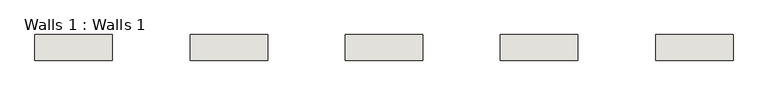
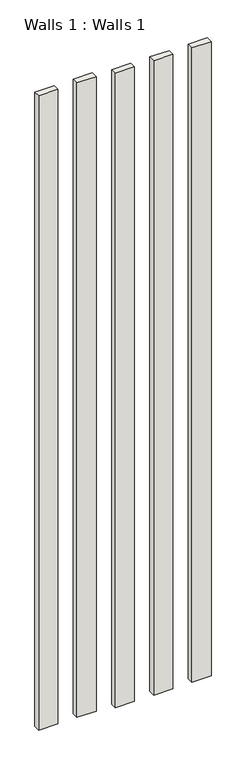
"""IFC4 building model written with IfcOpenShell, lengths in millimetres: wall geometry, Walls 1 : Walls 1."""

from ifc_helpers import new_model, si_unit, frame, origin, place, context, project, spatial, polyline, outline, extrude, source, transform, mapped, element, save


def walls_1_walls_1_4968a21e(model_context):
    return source(origin(), model_context, "Body", "SweptSolid", [
        extrude(outline(polyline([(-9508.1808238, -4092.3891189), (-9660.5808238, -4092.3891189), (-9660.5808238, -4041.5891189), (-9508.1808238, -4041.5891189), (-9508.1808238, -4092.3891189)])), frame((0.0, 0.0, 889.0), z_axis=(0.0, 0.0, 1.0), x_axis=(1.0, 0.0, 0.0)), (0.0, 0.0, 1.0), 5334.0),
        extrude(outline(polyline([(-9812.9808238, -4092.3891189), (-9965.3808238, -4092.3891189), (-9965.3808238, -4041.5891189), (-9812.9808238, -4041.5891189), (-9812.9808238, -4092.3891189)])), frame((0.0, 0.0, 889.0), z_axis=(0.0, 0.0, 1.0), x_axis=(1.0, 0.0, 0.0)), (0.0, 0.0, 1.0), 5334.0),
        extrude(outline(polyline([(-10422.5808238, -4092.3891189), (-10574.9808238, -4092.3891189), (-10574.9808238, -4041.5891189), (-10422.5808238, -4041.5891189), (-10422.5808238, -4092.3891189)])), frame((0.0, 0.0, 914.4), z_axis=(0.0, 0.0, 1.0), x_axis=(1.0, 0.0, 0.0)), (0.0, 0.0, 1.0), 5334.0),
        extrude(outline(polyline([(-10117.7808238, -4092.3891189), (-10270.1808238, -4092.3891189), (-10270.1808238, -4041.5891189), (-10117.7808238, -4041.5891189), (-10117.7808238, -4092.3891189)])), frame((0.0, 0.0, 889.0), z_axis=(0.0, 0.0, 1.0), x_axis=(1.0, 0.0, 0.0)), (0.0, 0.0, 1.0), 5334.0),
        extrude(outline(polyline([(-10727.3808238, -4092.3891189), (-10879.7808238, -4092.3891189), (-10879.7808238, -4041.5891189), (-10727.3808238, -4041.5891189), (-10727.3808238, -4092.3891189)])), frame((0.0, 0.0, 914.4), z_axis=(0.0, 0.0, 1.0), x_axis=(1.0, 0.0, 0.0)), (0.0, 0.0, 1.0), 5334.0),
    ])


if __name__ == "__main__":
    model = new_model("IFC4")
    model_context = context("Model", 3, world=origin())
    ifc_project = project(units=[si_unit("LENGTHUNIT", "METRE", prefix="MILLI")], contexts=[model_context])
    site = spatial("IfcSite", under=ifc_project)
    building = spatial("IfcBuilding", under=site)
    placement = place(None, origin())
    walls_1_walls_1_shape = walls_1_walls_1_4968a21e(model_context)
    element("IfcWall", 1, ObjectType="Walls 1 : Walls 1", at=placement, inside=building, context=model_context, shape_type="MappedRepresentation", body=[
        mapped(walls_1_walls_1_shape, transform((0.0, 0.0, 0.0), x_axis=(1.0, 0.0, 0.0), y_axis=(0.0, 1.0, 0.0), z_axis=(0.0, 0.0, 1.0))),
    ])
    save(model, "model.ifc")

# Revit data of these elements
# Element 1 (IfcWall, "Walls 1 : Walls 1")
#   Materials on its faces: "DESIGN"
# Materials
#   "DESIGN": class "Generic", colour RGB 255 214 0, transparency 0, Cost = 0
